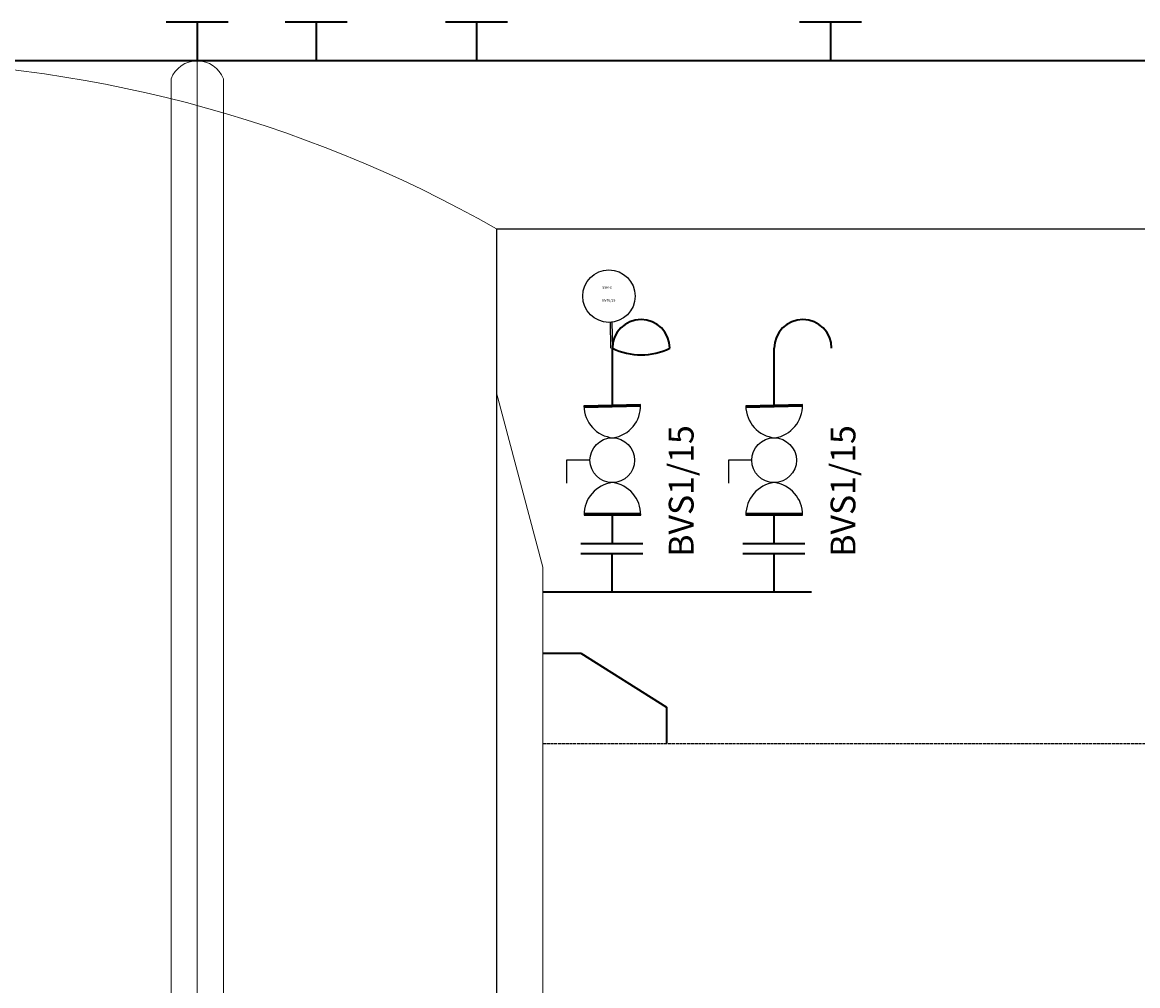
# Model space of a CAD drawing. Units: millimetres. Extents: x 353872 to 441597, y 126154 to 187356.
# Tile 10 of 28: x 394852 to 399262, y 145472 to 149281. Entities that reach past the tile are written whole.
import ezdxf

# ---------------------------------------------------------------- set-up
doc = ezdxf.new("R2010")
doc.units = ezdxf.units.MM
doc.linetypes.add('ACAD_ISO02W100', pattern=[15, 12, -3])
for name, color, linetype, lineweight in [('A-ANNO-DIMS', 2, 'Continuous', 18), ('P-ANNO-TEXT', 7, 'Continuous', 25), ('P-BNDY', 4, 'ACAD_ISO02W100', 25), ('P-INST', 6, 'Continuous', 25), ('P-INST-SIGN', 4, 'Continuous', 18), ('P-PIPE', 3, 'Continuous', 35), ('P-VALV', 2, 'Continuous', 25)]:
    doc.layers.add(name, color=color, linetype=linetype, lineweight=lineweight)
doc.styles.get("Standard").update_dxf_attribs({"font": 'arial.ttf'})
doc.dimstyles.get("Standard").update_dxf_attribs({"dimtxt": 0.18, "dimasz": 0.18, "dimexe": 0.18, "dimexo": 0.0625, "dimgap": 0.09, "dimtad": 0, "dimtih": 1, "dimtoh": 1, "dimdec": 4, "dimzin": 0, "dimdsep": 46, "dimtxsty": 'Standard', "dimcen": 0.09, "dimadec": 0, "dimazin": 0, "dimtfac": 1, "dimtdec": 4, "dimtofl": 0, "dimtmove": 0, "dimatfit": 3, "dimfxl": 1, "dimtolj": 1, "dimtzin": 0, "dimarcsym": 0})

# ---------------------------------------------------------------- blocks, each defined once
blk = doc.blocks.new('VALVE-C')
for points in [[(0, 2.6), (0, 0), (224, 0), (224, 3.5)], [(0, 2.5), (0, 2.5), (221.5, 2.5), (224, 2.5)], [(0.1, 5.1), (224, 5.1)], [(0.2, 7.8), (223.9, 7.8)]]:
    blk.add_lwpolyline(points)
for centre, radius, start, end in [((128.5, 1.3), 128.5, 97.3612, 180.5798), ((96.1, 1.7), 128, 359.2193, 82.8397)]:
    blk.add_arc(centre, radius, start, end)
blk = doc.blocks.new('*D29')
at = {"layer": 'A-ANNO-DIMS', "color": 0, "lineweight": -2, "transparency": 16777216}
for p, q in [((391689.9, 148464.5), (391689.9, 133812.7)), ((396727.5, 148464.5), (396727.5, 133812.7)), ((391690.1, 133812.8), (394208.4, 133812.8)), ((396727.3, 133812.8), (394209.1, 133812.8))]:
    blk.add_line(p, q, dxfattribs=at)
at = {"layer": 'A-ANNO-DIMS', "color": 0, "transparency": 16777216}
for points in [[(391690.1, 133812.9), (391690.1, 133812.8), (391689.9, 133812.8)], [(396727.3, 133812.9), (396727.3, 133812.8), (396727.5, 133812.8)]]:
    blk.add_solid(points, dxfattribs=at)
at = {"layer": 'Defpoints', "color": 0, "transparency": 16777216}
for p in [(391689.9, 148464.5), (396727.5, 148464.5), (396727.5, 133812.8)]:
    blk.add_point(p, dxfattribs=at)
at = {"layer": 'A-ANNO-DIMS', "color": 0, "transparency": 16777216, "insert": (394208.7, 133812.8), "char_height": 0.18, "attachment_point": 5}
blk.add_mtext('\\A1;5038', dxfattribs=at)
blk = doc.blocks.new('*D30')
at = {"layer": 'A-ANNO-DIMS', "color": 0, "lineweight": -2, "transparency": 16777216}
for p, q in [((396727.6, 148464.5), (440591.2, 148464.5)), ((440591, 148464.3), (440591, 145075.4)), ((440591, 141686), (440591, 145075)), ((396727.6, 141685.8), (440591.2, 141685.8))]:
    blk.add_line(p, q, dxfattribs=at)
at = {"layer": 'A-ANNO-DIMS', "color": 0, "transparency": 16777216}
for points in [[(440591, 148464.3), (440591, 148464.3), (440591, 148464.5)], [(440591, 141686), (440591, 141686), (440591, 141685.8)]]:
    blk.add_solid(points, dxfattribs=at)
at = {"layer": 'Defpoints', "color": 0, "transparency": 16777216}
for p in [(396727.5, 148464.5), (396727.5, 141685.8), (440591, 141685.8)]:
    blk.add_point(p, dxfattribs=at)
at = {"layer": 'A-ANNO-DIMS', "color": 0, "transparency": 16777216, "insert": (440591, 145075.2), "char_height": 0.18, "attachment_point": 5}
blk.add_mtext('\\A1;6779', dxfattribs=at)

msp = doc.modelspace()

# ---------------------------------------------------------------- linework, layer by layer
at = {"layer": 'P-BNDY'}
msp.add_line((396910.35, 146429.42), (434124.06, 146429.42), dxfattribs=at)
at = {"layer": 'P-INST'}
for p, q in [((397176.27, 148095.48), (397178.06, 147992.05)), ((397183.33, 148095.6), (397185.13, 147992.17))]:
    msp.add_line(p, q, dxfattribs=at)
msp.add_circle((397171.45, 148197.89), 103.68, dxfattribs=at)
at = {"layer": 'P-INST-SIGN'}
for p, q in [((395543.84, 149129.17), (395543.84, 142318.92)), ((395440.46, 149056.78), (395440.46, 142660.1)), ((395647.23, 149056.78), (395647.23, 142660.1)), ((396910.35, 147126.17), (396727.53, 147816.11))]:
    msp.add_line(p, q, dxfattribs=at)
for points in [[(396727.53, 148464.52), (396727.53, 148464.52), (396727.53, 141685.82)], [(396910.35, 147126.17), (396910.35, 141662.82)]]:
    msp.add_lwpolyline(points, dxfattribs=at)
for centre, radius, start, end in [((394208.72, 144024.11), 5105.06, 60.436, 119.564), ((395543.84, 149018.14), 110.37, 20.49642, 159.50358)]:
    msp.add_arc(centre, radius, start, end, dxfattribs=at)
at = {"layer": 'P-PIPE'}
for p, q in [((395666.22, 149280.57), (395421.46, 149280.57)), ((395543.84, 149280.57), (395543.84, 149129.17)), ((396136.94, 149280.57), (395892.18, 149280.57)), ((396014.56, 149280.57), (396014.56, 149129.17)), ((396770.53, 149280.57), (396525.77, 149280.57)), ((396648.15, 149280.57), (396648.15, 149129.17)), ((398169.84, 149280.57), (397925.08, 149280.57)), ((398047.46, 149280.57), (398047.46, 149129.17)), ((386450.69, 149129.17), (407087.67, 149129.17)), ((397185.13, 147766.4), (397185.13, 147992.17)), ((397824.82, 147766.4), (397824.82, 147992.17)), ((397183.87, 147332.29), (397183.87, 147218.88)), ((397823.56, 147332.29), (397823.56, 147218.88)), ((397305.59, 147218.88), (397060.83, 147218.88)), ((397945.28, 147218.88), (397700.52, 147218.88)), ((397305.59, 147179.72), (397060.83, 147179.72)), ((397183.21, 147179.72), (397183.21, 147028.32)), ((397945.28, 147179.72), (397700.52, 147179.72)), ((397822.9, 147179.72), (397822.9, 147028.32)), ((396910.35, 147028.32), (397972.62, 147028.32)), ((396910.35, 146785.93), (397060.81, 146785.93)), ((397060.81, 146785.93), (397399.6, 146572.79)), ((397399.6, 146572.79), (397399.6, 146429.42))]:
    msp.add_line(p, q, dxfattribs=at)
for centre, radius, start, end in [((397298.72, 147992.17), 113.59, 0, 180), ((397938.41, 147992.17), 113.59, 0, 180), ((397298.72, 148222.34), 256.67, 243.73283, 296.26717)]:
    msp.add_arc(centre, radius, start, end, dxfattribs=at)
at = {"layer": 'P-VALV'}
for points in [[(397096.54, 147549.34), (397004.09, 147549.34), (397004.09, 147458.58)], [(397736.23, 147549.34), (397643.78, 147549.34), (397643.78, 147458.58)]]:
    msp.add_lwpolyline(points, dxfattribs=at)
for centre in [(397184.83, 147549.34), (397824.52, 147549.34)]:
    msp.add_circle(centre, 88.29, dxfattribs=at)

# ---------------------------------------------------------------- block references
at = {"layer": 'P-VALV', "rotation": 181.30191700234}
for p in [(397296.65, 147768.94), (397936.35, 147768.94)]:
    msp.add_blockref('VALVE-C', p, dxfattribs=at)
at = {"layer": 'P-VALV'}
for p in [(397073.11, 147332.29), (397712.8, 147332.29)]:
    msp.add_blockref('VALVE-C', p, dxfattribs=at)

# ---------------------------------------------------------------- texts
at = {"layer": 'P-ANNO-TEXT'}
for s, p in [('SSR-3', (397145.43, 148227.48)), ('BVF6/25', (397145.43, 148176.36))]:
    msp.add_text(s, height=9.835, dxfattribs=at).set_placement(p)
for p in [(397506.13, 147167.74), (398145.83, 147167.74)]:
    msp.add_text('BVS1/15', height=98.09, rotation=90, dxfattribs=at).set_placement(p)

# ---------------------------------------------------------------- dimensions: what is measured, and where the dimension line sits
at = {"layer": 'A-ANNO-DIMS'}
dim = msp.add_linear_dim(base=(396727.53, 133812.84), p1=(391689.9, 148464.52), p2=(396727.53, 148464.52), dimstyle='Standard', override={"dimdec": 0, "dimlfac": 1, "dimrnd": 0, "dimzin": 0, "dimdsep": 46, "dimlunit": 2}, dxfattribs=at)
dim.commit()
dim.dimension.update_dxf_attribs({"geometry": '*D29', "text_midpoint": (394208.72, 133812.84)})
dim = msp.add_linear_dim(base=(440591, 141685.82), p1=(396727.53, 148464.52), p2=(396727.53, 141685.82), angle=90, dimstyle='Standard', override={"dimdec": 0, "dimlfac": 1, "dimrnd": 0, "dimzin": 0, "dimdsep": 46, "dimlunit": 2}, dxfattribs=at)
dim.commit()
dim.dimension.update_dxf_attribs({"geometry": '*D30', "text_midpoint": (440591, 145075.17)})

doc.saveas('drawing.dxf')
